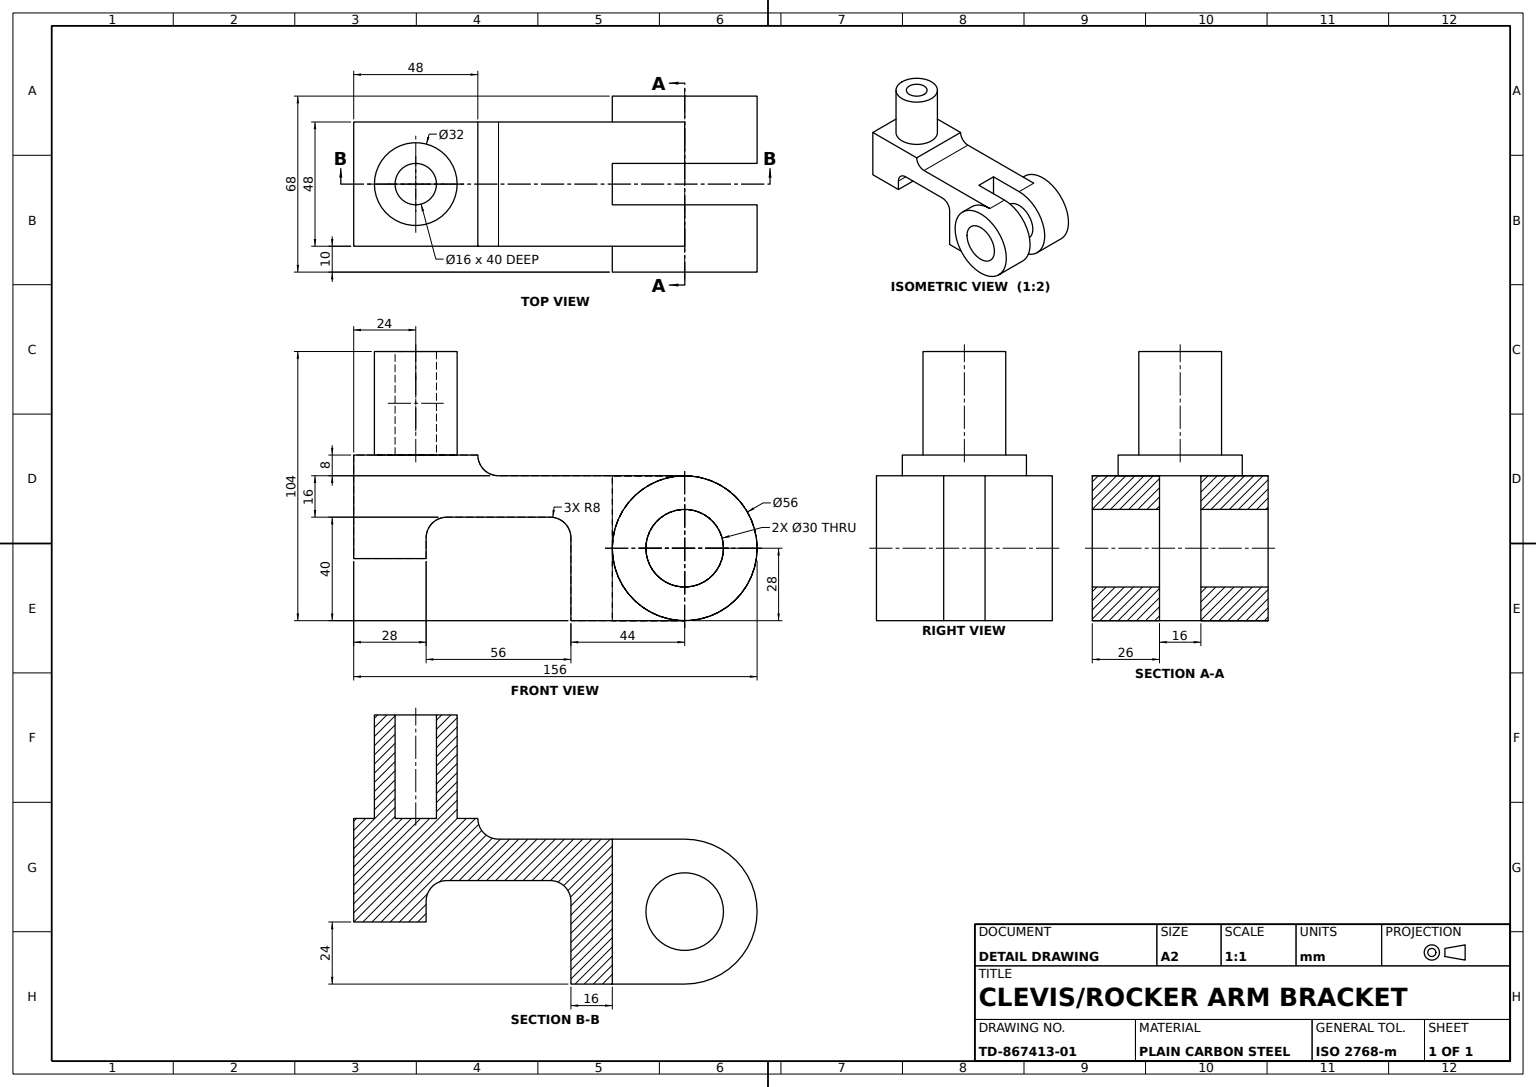
from build123d import *

# Parameters (mm, degrees)
ARM_BODY_DEPTH          = 24
BUSHING_BOSS_SKETCH_R   = 16
BUSHING_BOSS_SKETCH_R_2 = 8
BUSHING_BOSS_32_DEPTH   = 40
PIVOT_LUG_SKETCH_R      = 28
PIVOT_LUG_56_DEPTH      = 34
CLEVIS_SLOT_SKETCH_W    = 56
CLEVIS_SLOT_SKETCH_H    = 16
CLEVIS_SLOT_16MM_DEPTH  = 170.198108736
PIVOT_BORE_30_D         = 30


with BuildPart() as part:
    # Arm Profile Sketch → Arm Body (new, symmetric)
    with BuildSketch(Plane.XY):
        with BuildLine():
            Line((0, 0), (28, 0))
            Line((28, 0), (28, 8))
            ThreePointArc((28, 8), (30.343145751, 13.656854249), (36, 16))
            Line((36, 16), (76, 16))
            ThreePointArc((76, 16), (81.656854249, 13.656854249), (84, 8))
            Line((84, 8), (84, -24))
            Line((84, -24), (128, -24))
            Line((128, -24), (128, 32))
            Line((128, 32), (56, 32))
            ThreePointArc((56, 32), (50.343145751, 34.343145751), (48, 40))
            Line((48, 40), (0, 40))
            Line((0, 40), (0, 0))
        make_face()
    extrude(amount=ARM_BODY_DEPTH, both=True)

    # Bushing Boss Sketch → Bushing Boss Ø32 (add)
    with BuildSketch(Plane(origin=(0, 40, 0), x_dir=(1, 0, 0), z_dir=(0, 1, 0))):
        with Locations((24, 0)):
            Circle(BUSHING_BOSS_SKETCH_R)
        with Locations(Location((24, 0, 0), (0, 0, 180))):
            Circle(BUSHING_BOSS_SKETCH_R_2, mode=Mode.SUBTRACT)
    extrude(amount=BUSHING_BOSS_32_DEPTH)

    # Pivot Lug Sketch → Pivot Lug Ø56 (add, symmetric)
    with BuildSketch(Plane.XY):
        with Locations((128, 4)):
            Circle(PIVOT_LUG_SKETCH_R)
    extrude(amount=PIVOT_LUG_56_DEPTH, both=True)

    # Clevis Slot Sketch → Clevis Slot 16mm (cut, through all)
    with BuildSketch(Plane(origin=(0, 32, 0), x_dir=(1, 0, 0), z_dir=(0, 1, 0))):
        with Locations((128, 0)):
            Rectangle(CLEVIS_SLOT_SKETCH_W, CLEVIS_SLOT_SKETCH_H)
    extrude(amount=-CLEVIS_SLOT_16MM_DEPTH, mode=Mode.SUBTRACT)

    # Pivot Bore Ø30 (through all)
    with Locations(Plane.XY.offset(34)):
        with Locations((128, 4)):
            Hole(PIVOT_BORE_30_D / 2)


solid = part.part
